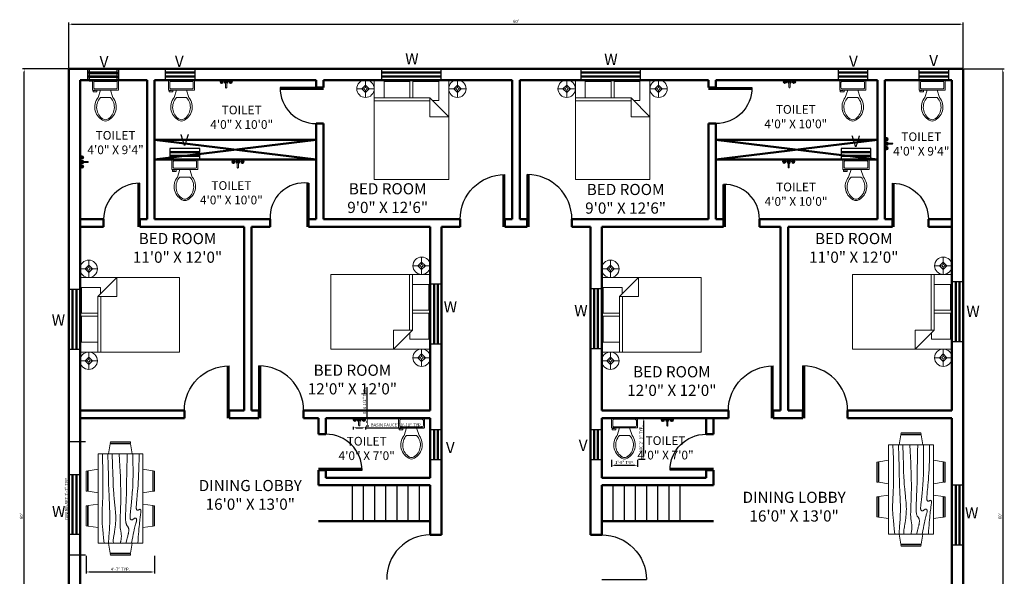
# Model space of a CAD drawing. Units: inches. Extents: x 2663 to 4539, y 2314 to 3111.
# Tile 2 of 4: x 2663 to 3456, y 2663 to 3111. Entities that reach past the tile are written whole.
import ezdxf

# ---------------------------------------------------------------- set-up
doc = ezdxf.new("R2010")
doc.units = ezdxf.units.IN
for name, color, linetype, lineweight in [('A-ANNO-DIMS', 2, 'Continuous', 18), ('A-ANNO-TEXT', 7, 'Continuous', 18), ('A-AREA-IDEN', 3, 'Continuous', 25), ('A-DOOR', 4, 'Continuous', 25), ('A-FLOR-FIXT', 8, 'Continuous', 18), ('A-FLOR-STRS', 2, 'Continuous', 25), ('A-FURN', 8, 'Continuous', 18), ('A-GLAZ', 3, 'Continuous', 25), ('A-WALL', 7, 'Continuous', 50)]:
    doc.layers.add(name, color=color, linetype=linetype, lineweight=lineweight)
doc.styles.get("Standard").update_dxf_attribs({"font": 'arial.ttf'})
doc.dimstyles.new('ISO-25', dxfattribs={"dimtxt": 2.5, "dimasz": 2.5, "dimexe": 1.25, "dimexo": 0.625, "dimtad": 1, "dimdec": 0, "dimlunit": 3, "dimtxsty": 'Standard', "dimcen": 2.5, "dimadec": 0, "dimazin": 0, "dimtfac": 1, "dimtdec": 0, "dimtmove": 0, "dimatfit": 3, "dimfxl": 1, "dimarcsym": 0})

# ---------------------------------------------------------------- blocks, each defined once
blk = doc.blocks.new('Bed - Queen')
for p, q in [((0, -80.00003), (0, 0)), ((0, 0), (59.99999, 0)), ((59.99999, 0), (59.99999, -80.00003)), ((7.99999, -1.2), (28.79998, -1.2)), ((7.99999, -14.4), (7.99999, -1.2)), ((28.79998, -1.2), (28.79998, -14.4)), ((31.19999, -1.2), (51.99999, -1.2)), ((31.19999, -14.4), (31.19999, -1.2)), ((51.99999, -1.2), (51.99999, -16.4)), ((0, -14.4), (44.8, -14.4)), ((59.99999, -29.6), (44.8, -14.4)), ((44.8, -14.4), (44.8, -29.6)), ((44.8, -16.8), (0, -16.8)), ((51.99999, -16.4), (46.79936, -16.4)), ((44.8, -29.6), (59.99999, -29.6)), ((59.99999, -80.00003), (0, -80.00003))]:
    blk.add_line(p, q)
blk = doc.blocks.new('Lamp - Table')
for p, q in [((-1, 0), (-7, 0)), ((0, 3), (-3, 0)), ((-3, 0), (0, -3)), ((0, 7), (0, 1)), ((3, 0), (0, 3)), ((0, -3), (3, 0)), ((1, 0), (7, 0)), ((0, -1), (0, -7))]:
    blk.add_line(p, q)
for radius in [7, 1]:
    blk.add_circle((0, 0), radius)
blk = doc.blocks.new('Toilet - top')
for p, q in [((9.5, -6), (9.5, -2)), ((-10, -8.5), (-8, -8.5)), ((-10, -9.5), (-10, -8.5)), ((-7, -9.5), (-10, -9.5)), ((-8, -8.5), (-8, -8)), ((-7, -8), (-7, -9.5)), ((-4, -8), (-6, -14)), ((4, -14), (-4, -14)), ((4, -8), (6, -14))]:
    blk.add_line(p, q)
blk.add_lwpolyline([(10.5, -8), (10.5, 0), (-10.5, 0), (-10.5, -8)], close=True)
for points in [[(-9.5, -2), (-9.5, -6)], [(8.5, -1), (-8.5, -1)], [(-8.5, -7), (8.5, -7)]]:
    blk.add_lwpolyline(points)
for centre, radius, start, end in [((-8.62, -1.88), 0.884, 81.8699, 188.1301), ((-8.62, -6.12), 0.884, 171.8699, 278.1301), ((8.62, -1.88), 0.884, 351.8699, 98.1301), ((8.62, -6.12), 0.884, 261.8699, 8.1301), ((3.52, -21.58), 12.17, 141.46911, 247.97143), ((4.2, -21.82), 11.33, 136.36773, 238.94682), ((-3.52, -21.58), 12.17, 292.02843, 38.53071), ((-4.2, -21.82), 11.33, 301.05301, 43.63209), ((0, -27.88), 4, 245.73182, 294.26817), ((0, -29), 4, 254.86053, 285.13947)]:
    blk.add_arc(centre, radius, start, end)
blk = doc.blocks.new('Dining Set - 36 x 72 in.')
for p, q in [((-22.2343, 26.00059), (-23.4847, 17.99762)), ((-22.2304, 26), (-5.7608, 26)), ((-22, 27.5), (-22.1562, 26.50042)), ((-5.8416, 26.5), (-22.1534, 26.5)), ((-22, 27.5), (-6, 27.5)), ((-5.8437, 26.49966), (-6, 27.5)), ((-4.5152, 17.99762), (-5.7655, 25.99926)), ((5.7657, 26.00059), (4.5153, 17.99762)), ((5.7696, 26), (22.2392, 26)), ((6, 27.5), (5.8438, 26.50042)), ((22.1584, 26.5), (5.8466, 26.5)), ((6, 27.5), (22, 27.5)), ((22.1563, 26.49966), (22, 27.5)), ((23.4848, 17.99762), (22.2345, 25.99926)), ((36, 18), (-36, 18)), ((-36, 18), (-36, -18)), ((36, -18), (36, 18)), ((-45.5, 8), (-44.5004, 8.15617)), ((-45.5, 8), (-45.5, -8)), ((-44.5, -8.15843), (-44.5, 8.15338)), ((-44.0006, 8.23428), (-35.9976, 9.48474)), ((-44, 8.23041), (-44, -8.23915)), ((44.0006, 8.23428), (35.9976, 9.48474)), ((44, 8.23041), (44, -8.23915)), ((44.5, -8.15843), (44.5, 8.15338)), ((45.5, 8), (44.5005, 8.15617)), ((45.5, 8), (45.5, -8)), ((-44.4997, -8.15631), (-45.5, -8)), ((-35.9976, -9.48476), (-43.9993, -8.2345)), ((35.9976, -9.48476), (43.9993, -8.2345)), ((44.4997, -8.15631), (45.5, -8)), ((-36, -18), (36, -18)), ((-22.2343, -26.0006), (-23.4847, -17.99762)), ((-4.5152, -17.99762), (-5.7655, -25.99928)), ((5.7657, -26.0006), (4.5153, -17.99762)), ((23.4848, -17.99762), (22.2345, -25.99928)), ((-22.2304, -26), (-5.7608, -26)), ((-22, -27.5), (-22.1562, -26.50044)), ((-5.8416, -26.5), (-22.1534, -26.5)), ((-22, -27.5), (-6, -27.5)), ((-5.8437, -26.49967), (-6, -27.5)), ((5.7696, -26), (22.2392, -26)), ((6, -27.5), (5.8438, -26.50044)), ((22.1584, -26.5), (5.8466, -26.5)), ((6, -27.5), (22, -27.5)), ((22.1563, -26.49967), (22, -27.5))]:
    blk.add_line(p, q)
for points in [[(-36, 15), (-31.1772, 14.97754), (-26.8079, 14.91406), (-22.8538, 14.81543), (-19.276, 14.6875), (-16.0362, 14.53613), (-13.0957, 14.36718), (-10.4159, 14.18652), (-7.9583, 14), (-5.6904, 13.81315), (-3.6035, 13.63021), (-1.6954, 13.45508), (0.0365, 13.29166), (1.5945, 13.14388), (2.9811, 13.01562), (4.1988, 12.9108), (5.25, 12.83333), (6.1393, 12.78613), (6.8802, 12.76823), (7.4883, 12.77767), (7.9792, 12.8125), (8.3685, 12.87077), (8.6719, 12.95052), (8.9049, 13.0498), (9.0833, 13.16666), (9.2205, 13.29899), (9.3216, 13.44401), (9.3895, 13.59879), (9.4271, 13.76041), (9.4373, 13.92594), (9.4232, 14.09245), (9.3875, 14.257), (9.3333, 14.41666), (9.2638, 14.56917), (9.1836, 14.71484), (9.0975, 14.85465), (9.0104, 14.98958), (8.9272, 15.1206), (8.8529, 15.2487), (8.7922, 15.37483), (8.75, 15.5), (8.7305, 15.62467), (8.7344, 15.74739), (8.7617, 15.86621), (8.8125, 15.97916), (8.8867, 16.08431), (8.9844, 16.17968), (9.1055, 16.26334), (9.25, 16.33333), (9.4189, 16.38802), (9.6172, 16.42708), (9.8506, 16.45052), (10.125, 16.45833), (10.4463, 16.45052), (10.8203, 16.42708), (11.2529, 16.38802), (11.75, 16.33333), (12.3184, 16.26318), (12.9694, 16.17838), (13.7151, 16.07991), (14.5677, 15.96875), (15.5395, 15.84586), (16.6426, 15.71224), (17.8893, 15.56884), (19.2917, 15.41666), (20.859, 15.25667), (22.5879, 15.08984), (24.4721, 14.91715), (26.5052, 14.73958), (28.6809, 14.5581), (30.9929, 14.3737), (33.4347, 14.18733), (36, 14)], [(-36, 10), (-28.9766, 10.14274), (-23.1725, 10.20442), (-18.4241, 10.19775), (-14.5677, 10.13541), (-11.4399, 10.03011), (-8.877, 9.89453), (-6.7154, 9.74137), (-4.7917, 9.58333), (-2.9698, 9.43082), (-1.2246, 9.28515), (0.4415, 9.14534), (2.026, 9.01041), (3.5266, 8.87939), (4.9408, 8.7513), (6.266, 8.62516), (7.5, 8.5), (8.6411, 8.37549), (9.6914, 8.2539), (10.6538, 8.13818), (11.5312, 8.03125), (12.3267, 7.93603), (13.043, 7.85547), (13.6831, 7.79248), (14.25, 7.75), (14.7471, 7.7303), (15.1797, 7.73307), (15.5537, 7.75732), (15.875, 7.80208), (16.1494, 7.86637), (16.3828, 7.94922), (16.5811, 8.04964), (16.75, 8.16666), (16.8944, 8.29915), (17.0143, 8.44531), (17.1089, 8.60319), (17.1771, 8.77083), (17.218, 8.94629), (17.2305, 9.1276), (17.2137, 9.31282), (17.1667, 9.5), (17.0895, 9.6875), (16.987, 9.875), (16.8649, 10.0625), (16.7292, 10.25), (16.5856, 10.4375), (16.4401, 10.625), (16.2985, 10.8125), (16.1667, 11), (16.05, 11.18733), (15.9518, 11.3737), (15.8752, 11.5581), (15.8229, 11.73958), (15.798, 11.91715), (15.8034, 12.08984), (15.842, 12.25667), (15.9167, 12.41666), (16.0295, 12.56836), (16.1784, 12.70833), (16.3605, 12.83268), (16.5729, 12.9375), (16.8127, 13.01888), (17.0768, 13.07291), (17.3625, 13.0957), (17.6667, 13.08333), (17.9894, 13.03312), (18.3418, 12.94726), (18.7382, 12.82918), (19.1927, 12.68229), (19.7195, 12.51001), (20.3327, 12.31575), (21.0465, 12.10294), (21.875, 11.875), (22.8357, 11.63354), (23.959, 11.37304), (25.2786, 11.08618), (26.8282, 10.76562), (28.6414, 10.40405), (30.752, 9.99414), (33.1936, 9.52856), (36, 9)], [(-36, 5.5), (-30.7157, 5.3348), (-26.069, 5.20963), (-21.9946, 5.11767), (-18.4271, 5.05208), (-15.3009, 5.00602), (-12.5508, 4.97265), (-10.1112, 4.94515), (-7.9167, 4.91666), (-5.909, 4.88167), (-4.0586, 4.83984), (-2.3429, 4.79215), (-0.7396, 4.73958), (0.7739, 4.6831), (2.22, 4.6237), (3.6213, 4.56233), (5, 4.5), (6.373, 4.43782), (7.7344, 4.3776), (9.0723, 4.32129), (10.375, 4.27083), (11.6309, 4.22819), (12.8281, 4.19531), (13.9551, 4.17415), (15, 4.16666), (15.954, 4.17448), (16.819, 4.19791), (17.6001, 4.23698), (18.3021, 4.29166), (18.9299, 4.36198), (19.4883, 4.44791), (19.9823, 4.54948), (20.4167, 4.66666), (20.7969, 4.79899), (21.1302, 4.94401), (21.4245, 5.09879), (21.6875, 5.26041), (21.9271, 5.42594), (22.1511, 5.59245), (22.3672, 5.757), (22.5834, 5.91666), (22.8065, 6.06868), (23.0404, 6.21093), (23.2879, 6.34147), (23.5521, 6.45833), (23.8358, 6.55957), (24.142, 6.64323), (24.4735, 6.70735), (24.8334, 6.75), (25.2235, 6.76969), (25.642, 6.76692), (26.0858, 6.74267), (26.5521, 6.69791), (27.0379, 6.63362), (27.5404, 6.55078), (28.0565, 6.45036), (28.5834, 6.33333), (29.1242, 6.19987), (29.7071, 6.04687), (30.3661, 5.87044), (31.1354, 5.66666), (32.0493, 5.43164), (33.142, 5.16146), (34.4475, 4.85221), (36, 4.5)], [(-36, -1), (-30.7915, -0.6591), (-26.0195, -0.38216), (-21.6519, -0.16284), (-17.6563, 0.00521), (-14.0005, 0.12833), (-10.6523, 0.21289), (-7.5796, 0.26522), (-4.75, 0.29166), (-2.134, 0.29793), (0.2878, 0.28711), (2.5317, 0.26163), (4.6146, 0.22396), (6.5529, 0.17651), (8.3633, 0.12174), (10.0623, 0.06209), (11.6667, 0), (13.1899, -0.06201), (14.6341, -0.1211), (15.9982, -0.17432), (17.2813, -0.21875), (18.4823, -0.25147), (19.6003, -0.26953), (20.6343, -0.27002), (21.5834, -0.25), (22.4481, -0.20768), (23.2357, -0.14584), (23.9549, -0.06836), (24.6146, 0.02083), (25.2235, 0.11784), (25.7904, 0.21875), (26.3241, 0.31966), (26.8334, 0.41666), (27.3265, 0.50618), (27.8099, 0.58593), (28.2894, 0.65397), (28.7709, 0.70833), (29.2601, 0.74707), (29.763, 0.76823), (30.2855, 0.76985), (30.8334, 0.75), (31.4088, 0.70784), (31.9994, 0.64713), (32.589, 0.57275), (33.1615, 0.48958), (33.7008, 0.4025), (34.1908, 0.3164), (34.6153, 0.23616), (34.9584, 0.16666), (35.2099, 0.11165), (35.3848, 0.07031), (35.504, 0.04069), (35.5886, 0.02083), (35.6594, 0.00879), (35.7377, 0.0026), (35.8442, 0.00032), (36, 0)], [(-36, -6.5), (-27.1843, -6.31267), (-20.084, -6.1263), (-14.469, -5.9419), (-10.1094, -5.76042), (-6.7752, -5.58285), (-4.2363, -5.41016), (-2.2629, -5.24333), (-0.625, -5.08334), (0.8708, -4.93099), (2.2715, -4.78646), (3.5872, -4.64974), (4.8281, -4.52084), (6.0046, -4.39974), (7.127, -4.28646), (8.2053, -4.18099), (9.25, -4.08334), (10.2705, -3.99382), (11.2734, -3.91407), (12.2647, -3.84603), (13.25, -3.79167), (14.2354, -3.75293), (15.2266, -3.73177), (16.2295, -3.73015), (17.25, -3.75), (18.2912, -3.79248), (19.3451, -3.85547), (20.4009, -3.93604), (21.4479, -4.03125), (22.4754, -4.13819), (23.4727, -4.25391), (24.4289, -4.37549), (25.3334, -4.5), (26.1785, -4.62492), (26.9694, -4.74935), (27.7145, -4.87281), (28.4219, -4.99479), (29.1, -5.11483), (29.7572, -5.23242), (30.4016, -5.34709), (31.0417, -5.45834), (31.6837, -5.56437), (32.3262, -5.65821), (32.9658, -5.73153), (33.599, -5.77604), (34.2224, -5.78345), (34.8327, -5.74545), (35.4264, -5.65373), (36, -5.5)], [(-36, -10), (-26.4022, -9.81299), (-18.4675, -9.62891), (-11.9839, -9.45069), (-6.7396, -9.28125), (-2.5226, -9.12354), (0.8789, -8.98047), (3.6769, -8.85498), (6.0833, -8.75), (8.2767, -8.66765), (10.3021, -8.60677), (12.1712, -8.56543), (13.8958, -8.54167), (15.4876, -8.53353), (16.9583, -8.53907), (18.3197, -8.55632), (19.5834, -8.58334), (20.7616, -8.61841), (21.8685, -8.66081), (22.9188, -8.71004), (23.9271, -8.76563), (24.9081, -8.82707), (25.8763, -8.89388), (26.8465, -8.96558), (27.8334, -9.04167), (28.8474, -9.12118), (29.8828, -9.20117), (30.93, -9.27824), (31.9792, -9.34896), (33.0205, -9.40991), (34.0443, -9.45768), (35.0407, -9.48885), (36, -9.5)], [(-36, -14.5), (-30.0881, -14.33513), (-25.0332, -14.21224), (-20.7312, -14.12647), (-17.0781, -14.07292), (-13.97, -14.04671), (-11.3027, -14.04297), (-8.9724, -14.05681), (-6.875, -14.08334), (-4.9224, -14.11833), (-3.0905, -14.16016), (-1.3709, -14.20785), (0.2448, -14.26042), (1.7647, -14.3169), (3.1973, -14.3763), (4.5507, -14.43767), (5.8333, -14.5), (7.0554, -14.5621), (8.235, -14.62175), (9.3922, -14.67652), (10.5469, -14.72396), (11.7192, -14.76164), (12.929, -14.78711), (14.1965, -14.79794), (15.5417, -14.79167), (16.9933, -14.76424), (18.6152, -14.70508), (20.4804, -14.60197), (22.6615, -14.44271), (25.2312, -14.21509), (28.2624, -13.9069), (31.8277, -13.50594), (36, -13)]]:
    blk.add_lwpolyline(points)
blk = doc.blocks.new('Faucet - Bathroom top')
for p, q in [((-4.107, 0.125), (-4.375, 0.125)), ((-3.75, 0.4788), (-3.75, 0.75)), ((-3.5, 0.482), (-3.5, 0.75)), ((-3.1461, 0.125), (-2.875, 0.125)), ((3.143, 0.125), (2.875, 0.125)), ((3.5, 0.4788), (3.5, 0.75)), ((3.75, 0.482), (3.75, 0.75)), ((4.1039, 0.125), (4.375, 0.125)), ((-4.1039, -0.125), (-4.375, -0.125)), ((-3.75, -0.4821), (-3.75, -0.75)), ((-3.5, -0.4789), (-3.5, -0.75)), ((-3.143, -0.125), (-2.875, -0.125)), ((-0.5, -0.8639), (-0.5, -4.5)), ((0.5, -4.5), (0.5, -0.8631)), ((3.1461, -0.125), (2.875, -0.125)), ((3.5, -0.4821), (3.5, -0.75)), ((3.75, -0.4789), (3.75, -0.75)), ((4.107, -0.125), (4.375, -0.125))]:
    blk.add_line(p, q)
for centre, radius in [((-3.625, 0), 1.375), ((-4.625, 0), 0.2795), ((-3.625, 0), 0.5), ((-3.625, 1), 0.2795), ((-2.625, 0), 0.2795), ((0, 0), 0.5), ((3.625, 0), 1.375), ((2.625, 0), 0.2795), ((3.625, 0), 0.5), ((3.625, 1), 0.2795), ((4.625, 0), 0.2795), ((-3.625, -1), 0.2795), ((3.625, -1), 0.2795)]:
    blk.add_circle(centre, radius)
for centre, radius, start, end in [((-3.625, 0), 1, 105.2407, 164.2093), ((-3.625, 0), 1, 16.44125, 74.07887), ((0, 0), 1.5, 289.6514, 250.3603), ((0, 0), 1, 300.3431, 239.7554), ((3.625, 0), 1, 106.12, 164.0884), ((3.625, 0), 1, 16.23422, 73.90469), ((-3.625, 0), 1, 196.2342, 253.9047), ((-3.625, 0), 1, 286.12, 344.0884), ((0, -4.5), 0.5, 180, 0), ((3.625, 0), 1, 196.4413, 254.0789), ((3.625, 0), 1, 285.2407, 344.2093)]:
    blk.add_arc(centre, radius, start, end)
blk = doc.blocks.new('*D10')
at = {"layer": 'A-ANNO-DIMS', "color": 0, "lineweight": -2, "transparency": 16777216}
for p, q in [((2702.63, 3071.54), (2702.63, 3108.16)), ((3422.63, 3071.54), (3422.63, 3108.16)), ((2705.13, 3106.91), (3420.13, 3106.91))]:
    blk.add_line(p, q, dxfattribs=at)
at = {"layer": 'A-ANNO-DIMS', "color": 0, "transparency": 16777216}
for points in [[(2705.13, 3107.33), (2705.13, 3106.5), (2702.63, 3106.91)], [(3420.13, 3107.33), (3420.13, 3106.5), (3422.63, 3106.91)]]:
    blk.add_solid(points, dxfattribs=at)
at = {"layer": 'Defpoints', "color": 0, "transparency": 16777216}
for p in [(3422.63, 3106.91), (2702.63, 3070.91), (3422.63, 3070.91)]:
    blk.add_point(p, dxfattribs=at)
at = {"layer": 'A-ANNO-DIMS', "color": 0, "transparency": 16777216, "insert": (3062.63, 3108.82), "char_height": 2.5, "attachment_point": 5}
blk.add_mtext("60'", dxfattribs=at)
blk = doc.blocks.new('*D11')
at = {"layer": 'A-ANNO-DIMS', "color": 0, "lineweight": -2, "transparency": 16777216}
for p, q in [((3423.26, 3070.91), (3455.77, 3070.91)), ((3454.52, 3068.41), (3454.52, 2353.41)), ((3423.26, 2350.91), (3455.77, 2350.91))]:
    blk.add_line(p, q, dxfattribs=at)
at = {"layer": 'A-ANNO-DIMS', "color": 0, "transparency": 16777216}
for points in [[(3454.11, 3068.41), (3454.94, 3068.41), (3454.52, 3070.91)], [(3454.11, 2353.41), (3454.94, 2353.41), (3454.52, 2350.91)]]:
    blk.add_solid(points, dxfattribs=at)
at = {"layer": 'Defpoints', "color": 0, "transparency": 16777216}
for p in [(3422.63, 3070.91), (3422.63, 2350.91), (3454.52, 2350.91)]:
    blk.add_point(p, dxfattribs=at)
at = {"layer": 'A-ANNO-DIMS', "color": 0, "transparency": 16777216, "insert": (3452.62, 2710.91), "char_height": 2.5, "attachment_point": 5, "rotation": 90}
blk.add_mtext("60'", dxfattribs=at)
blk = doc.blocks.new('*D19')
at = {"layer": 'A-ANNO-DIMS', "color": 0, "lineweight": -2, "transparency": 16777216}
for p, q in [((2702.01, 3070.91), (2665.38, 3070.91)), ((2666.63, 2353.41), (2666.63, 3068.41)), ((2702.01, 2350.91), (2665.38, 2350.91))]:
    blk.add_line(p, q, dxfattribs=at)
at = {"layer": 'A-ANNO-DIMS', "color": 0, "transparency": 16777216}
for points in [[(2666.21, 3068.41), (2667.05, 3068.41), (2666.63, 3070.91)], [(2666.21, 2353.41), (2667.05, 2353.41), (2666.63, 2350.91)]]:
    blk.add_solid(points, dxfattribs=at)
at = {"layer": 'Defpoints', "color": 0, "transparency": 16777216}
for p in [(2666.63, 3070.91), (2702.63, 3070.91), (2702.63, 2350.91)]:
    blk.add_point(p, dxfattribs=at)
at = {"layer": 'A-ANNO-DIMS', "color": 0, "transparency": 16777216, "insert": (2664.73, 2710.91), "char_height": 2.5, "attachment_point": 5, "rotation": 90}
blk.add_mtext("60'", dxfattribs=at)
blk = doc.blocks.new('WIN-1200')
for p, q in [((0, 48), (0, 0)), ((9, 48), (0, 48)), ((0, 48), (0, 48)), ((9, 0), (9, 48)), ((0, 0), (9, 0))]:
    blk.add_line(p, q)
blk = doc.blocks.new('VENT-600')
for p, q in [((24, 9), (0, 9)), ((0, 9), (0, 0)), ((24, 0), (24, 9)), ((0, 0), (24, 0))]:
    blk.add_line(p, q)
blk = doc.blocks.new('DOOR-750')
blk.add_line((2901.63, 3055.91), (2872.63, 3055.91))
blk.add_arc((2901.63, 3055.91), 29, 180, 270)
blk = doc.blocks.new('DOOR-900')
blk.add_line((3071.63, 2949.91), (3071.63, 2985.91))
blk.add_arc((3071.63, 2949.91), 36, 0, 90)
blk = doc.blocks.new('*D32')
at = {"layer": 'A-ANNO-DIMS', "color": 0, "lineweight": -2, "transparency": 16777216}
for p, q in [((3161.16, 2789.91), (3166.74, 2789.91)), ((3165.49, 2759.37), (3165.49, 2787.41)), ((3161.16, 2756.87), (3166.74, 2756.87))]:
    blk.add_line(p, q, dxfattribs=at)
at = {"layer": 'A-ANNO-DIMS', "color": 0, "transparency": 16777216}
for points in [[(3165.07, 2787.41), (3165.91, 2787.41), (3165.49, 2789.91)], [(3165.07, 2759.37), (3165.91, 2759.37), (3165.49, 2756.87)]]:
    blk.add_solid(points, dxfattribs=at)
at = {"layer": 'Defpoints', "color": 0, "transparency": 16777216}
for p in [(3160.53, 2789.91), (3165.49, 2789.91), (3160.53, 2756.87)]:
    blk.add_point(p, dxfattribs=at)
at = {"layer": 'A-ANNO-DIMS', "color": 0, "transparency": 16777216, "insert": (3163.57, 2773.39), "char_height": 2.5, "attachment_point": 5, "rotation": 90}
blk.add_mtext('WC 2\'-9" TYP.', dxfattribs=at)
blk = doc.blocks.new('*D33')
at = {"layer": 'A-ANNO-DIMS', "color": 0, "lineweight": -2, "transparency": 16777216}
for p, q in [((3139.53, 2756.24), (3139.53, 2750.66)), ((3142.03, 2751.91), (3158.03, 2751.91)), ((3160.53, 2756.24), (3160.53, 2750.66))]:
    blk.add_line(p, q, dxfattribs=at)
at = {"layer": 'A-ANNO-DIMS', "color": 0, "transparency": 16777216}
for points in [[(3142.03, 2752.33), (3142.03, 2751.5), (3139.53, 2751.91)], [(3158.03, 2752.33), (3158.03, 2751.5), (3160.53, 2751.91)]]:
    blk.add_solid(points, dxfattribs=at)
at = {"layer": 'Defpoints', "color": 0, "transparency": 16777216}
for p in [(3139.53, 2756.87), (3160.53, 2756.87), (3160.53, 2751.91)]:
    blk.add_point(p, dxfattribs=at)
at = {"layer": 'A-ANNO-DIMS', "color": 0, "transparency": 16777216, "insert": (3150.03, 2753.81), "char_height": 2.5, "attachment_point": 5}
blk.add_mtext('1\'-9" TYP.', dxfattribs=at)
blk = doc.blocks.new('*D34')
at = {"layer": 'A-ANNO-DIMS', "color": 0, "lineweight": -2, "transparency": 16777216}
for p, q in [((2931.42, 2782.93), (2931.42, 2780.81)), ((2941.42, 2782.93), (2941.42, 2780.81)), ((2933.92, 2782.06), (2938.92, 2782.06)), ((2941.42, 2782.06), (2988.63, 2782.06))]:
    blk.add_line(p, q, dxfattribs=at)
at = {"layer": 'A-ANNO-DIMS', "color": 0, "transparency": 16777216}
for points in [[(2933.92, 2782.48), (2933.92, 2781.64), (2931.42, 2782.06)], [(2938.92, 2782.48), (2938.92, 2781.64), (2941.42, 2782.06)]]:
    blk.add_solid(points, dxfattribs=at)
at = {"layer": 'Defpoints', "color": 0, "transparency": 16777216}
for p in [(2931.42, 2783.56), (2941.42, 2783.56), (2941.42, 2782.06)]:
    blk.add_point(p, dxfattribs=at)
at = {"layer": 'A-ANNO-DIMS', "color": 0, "transparency": 16777216, "insert": (2966.28, 2783.98), "char_height": 2.5, "attachment_point": 5}
blk.add_mtext('BASIN FAUCET 0\'-10" TYP.', dxfattribs=at)
blk = doc.blocks.new('*D35')
at = {"layer": 'A-ANNO-DIMS', "color": 0, "lineweight": -2, "transparency": 16777216}
for p, q in [((2942.92, 2790.06), (2942.92, 2814.87)), ((2942.05, 2790.06), (2944.17, 2790.06)), ((2942.05, 2783.56), (2944.17, 2783.56)), ((2942.92, 2786.06), (2942.92, 2787.56))]:
    blk.add_line(p, q, dxfattribs=at)
at = {"layer": 'A-ANNO-DIMS', "color": 0, "transparency": 16777216}
for points in [[(2942.5, 2787.56), (2943.34, 2787.56), (2942.92, 2790.06)], [(2942.5, 2786.06), (2943.34, 2786.06), (2942.92, 2783.56)]]:
    blk.add_solid(points, dxfattribs=at)
at = {"layer": 'Defpoints', "color": 0, "transparency": 16777216}
for p in [(2941.42, 2790.06), (2941.42, 2783.56), (2942.92, 2790.06)]:
    blk.add_point(p, dxfattribs=at)
at = {"layer": 'A-ANNO-DIMS', "color": 0, "transparency": 16777216, "insert": (2941, 2803.72), "char_height": 2.5, "attachment_point": 5, "rotation": 90}
blk.add_mtext('0\'-6 1/2" TYP.', dxfattribs=at)
blk = doc.blocks.new('*D44')
at = {"layer": 'A-ANNO-DIMS', "color": 0, "lineweight": -2, "transparency": 16777216}
for p, q in [((2715.98, 2770.68), (2701.71, 2770.68)), ((2702.96, 2768.18), (2702.96, 2682.18)), ((2715.98, 2679.68), (2701.71, 2679.68))]:
    blk.add_line(p, q, dxfattribs=at)
at = {"layer": 'A-ANNO-DIMS', "color": 0, "transparency": 16777216}
for points in [[(2702.54, 2768.18), (2703.38, 2768.18), (2702.96, 2770.68)], [(2702.54, 2682.18), (2703.38, 2682.18), (2702.96, 2679.68)]]:
    blk.add_solid(points, dxfattribs=at)
at = {"layer": 'Defpoints', "color": 0, "transparency": 16777216}
for p in [(2716.61, 2770.68), (2702.96, 2679.68), (2716.61, 2679.68)]:
    blk.add_point(p, dxfattribs=at)
at = {"layer": 'A-ANNO-DIMS', "color": 0, "transparency": 16777216, "insert": (2701.04, 2725.18), "char_height": 2.5, "attachment_point": 5, "rotation": 90}
blk.add_mtext('DINING SET 7\'-7" TYP.', dxfattribs=at)
blk = doc.blocks.new('*D45')
at = {"layer": 'A-ANNO-DIMS', "color": 0, "lineweight": -2, "transparency": 16777216}
for p, q in [((2716.61, 2679.05), (2716.61, 2664.78)), ((2771.61, 2679.05), (2771.61, 2664.78)), ((2719.11, 2666.03), (2769.11, 2666.03))]:
    blk.add_line(p, q, dxfattribs=at)
at = {"layer": 'A-ANNO-DIMS', "color": 0, "transparency": 16777216}
for points in [[(2719.11, 2666.45), (2719.11, 2665.61), (2716.61, 2666.03)], [(2769.11, 2666.45), (2769.11, 2665.61), (2771.61, 2666.03)]]:
    blk.add_solid(points, dxfattribs=at)
at = {"layer": 'Defpoints', "color": 0, "transparency": 16777216}
for p in [(2716.61, 2679.68), (2771.61, 2679.68), (2771.61, 2666.03)]:
    blk.add_point(p, dxfattribs=at)
at = {"layer": 'A-ANNO-DIMS', "color": 0, "transparency": 16777216, "insert": (2744.11, 2667.91), "char_height": 2.5, "attachment_point": 5}
blk.add_mtext('4\'-7" TYP.', dxfattribs=at)

msp = doc.modelspace()

# ---------------------------------------------------------------- linework, layer by layer
at = {"layer": 'A-DOOR'}
for centre, radius, start, end in [((2892.16, 2951.55), 27.58, 82.77506, 183.40664), ((3230.63, 2949.91), 28, 360, 92.04671), ((2993.63, 2660.91), 35, 90, 181.63725)]:
    msp.add_arc(centre, radius, start, end, dxfattribs=at)
at = {"layer": 'A-FLOR-STRS'}
for p, q in [((2930.63, 2735.91), (2930.63, 2706.91)), ((2939.63, 2735.91), (2939.63, 2706.91)), ((2948.63, 2735.91), (2948.63, 2706.91)), ((2957.63, 2735.91), (2957.63, 2706.91)), ((2966.63, 2735.91), (2966.63, 2706.91)), ((2975.63, 2735.91), (2975.63, 2706.91)), ((2984.63, 2735.91), (2984.63, 2706.91)), ((3140.63, 2735.91), (3140.63, 2706.91)), ((3149.63, 2735.91), (3149.63, 2706.91)), ((3158.63, 2735.91), (3158.63, 2706.91)), ((3167.63, 2735.91), (3167.63, 2706.91)), ((3176.63, 2735.91), (3176.63, 2706.91)), ((3185.63, 2735.91), (3185.63, 2706.91)), ((3194.63, 2735.91), (3194.63, 2706.91))]:
    msp.add_line(p, q, dxfattribs=at)
at = {"layer": 'A-WALL'}
for p, q in [((2702.63, 3070.91), (3422.63, 3070.91)), ((2702.63, 2350.91), (2702.63, 3070.91)), ((3422.63, 3070.91), (3422.63, 2350.91)), ((2711.63, 3061.91), (2765.63, 3061.91)), ((2711.63, 2624.91), (2711.63, 3061.91)), ((2741.59, 3067.91), (2717.59, 3067.91)), ((2717.59, 3064.91), (2741.59, 3064.91)), ((2742.88, 3067.41), (2718.88, 3067.41)), ((2718.88, 3064.41), (2742.88, 3064.41)), ((2765.63, 2949.91), (2765.63, 3061.91)), ((2771.63, 2949.91), (2771.63, 3061.91)), ((2771.63, 3061.91), (2901.63, 3061.91)), ((2804.19, 3067.91), (2780.19, 3067.91)), ((2780.19, 3064.91), (2804.19, 3064.91)), ((2901.63, 3061.91), (2901.63, 3055.91)), ((2901.63, 3055.91), (2901.63, 3061.91)), ((2907.63, 3061.91), (3059.63, 3061.91)), ((2907.63, 3055.91), (2907.63, 3061.91)), ((3002.32, 3067.91), (2954.32, 3067.91)), ((2954.32, 3064.91), (3002.32, 3064.91)), ((3059.63, 2949.91), (3059.63, 3061.91)), ((3065.63, 3061.91), (3065.63, 2949.91)), ((3065.63, 3061.91), (3217.63, 3061.91)), ((3162.93, 3067.91), (3114.93, 3067.91)), ((3114.93, 3064.91), (3162.93, 3064.91)), ((3217.63, 3061.91), (3217.63, 3055.91)), ((3223.63, 3061.91), (3223.63, 3055.91)), ((3223.63, 3061.91), (3353.63, 3061.91)), ((3223.63, 3061.91), (3223.63, 3055.91)), ((3345.92, 3067.91), (3321.92, 3067.91)), ((3321.92, 3064.91), (3345.92, 3064.91)), ((3353.63, 3061.91), (3353.63, 2949.91)), ((3359.63, 3061.91), (3359.63, 2949.91)), ((3359.63, 3061.91), (3413.63, 3061.91)), ((3411.01, 3067.91), (3387.01, 3067.91)), ((3387.01, 3064.91), (3411.01, 3064.91)), ((3413.63, 3061.91), (3413.63, 2795.91)), ((2901.63, 3054.91), (2872.63, 3054.91)), ((2901.63, 3055.91), (2907.63, 3055.91)), ((2901.63, 3054.91), (2907.63, 3054.91)), ((3223.63, 3055.91), (3217.63, 3055.91)), ((3223.63, 3054.91), (3217.63, 3054.91)), ((3223.63, 3054.91), (3252.63, 3054.91)), ((2901.63, 2949.91), (2901.63, 3026.91)), ((2907.63, 3026.91), (2901.63, 3026.91)), ((2907.63, 2949.91), (2907.63, 3026.91)), ((3217.63, 3026.91), (3223.63, 3026.91)), ((3217.63, 3026.91), (3217.63, 2949.91)), ((3223.63, 3026.91), (3223.63, 2949.91)), ((2771.63, 3013.91), (2901.63, 3013.91)), ((2771.63, 3013.91), (2901.63, 2997.91)), ((2901.63, 3013.91), (2771.63, 2997.91)), ((2901.63, 2997.91), (2901.63, 3013.91)), ((3223.63, 3013.91), (3353.63, 3013.91)), ((3353.63, 3013.91), (3223.63, 2997.91)), ((3223.63, 2997.91), (3223.63, 3013.91)), ((3223.63, 3013.91), (3353.63, 2997.91)), ((2771.63, 2997.91), (2901.63, 2997.91)), ((2808.04, 3003.94), (2784.04, 3003.94)), ((2784.04, 3000.94), (2808.04, 3000.94)), ((3223.63, 2997.91), (3353.63, 2997.91)), ((3348.36, 3003.88), (3324.36, 3003.88)), ((3324.36, 3000.88), (3348.36, 3000.88)), ((3052.63, 2949.91), (3052.63, 2985.91)), ((3072.63, 2949.91), (3072.63, 2985.91)), ((2758.63, 2949.91), (2758.63, 2978.91)), ((2894.63, 2949.91), (2894.63, 2978.91)), ((2895.63, 2949.91), (2895.63, 2978.91)), ((3229.63, 2949.91), (3229.63, 2977.9)), ((3230.63, 2949.91), (3230.63, 2977.91)), ((3366.63, 2949.91), (3366.63, 2978.91)), ((2711.63, 2949.91), (2730.63, 2949.91)), ((2730.63, 2943.91), (2730.63, 2949.91)), ((2758.63, 2949.91), (2758.63, 2943.91)), ((2765.63, 2949.91), (2759.63, 2949.91)), ((2759.63, 2949.91), (2759.63, 2943.91)), ((2759.63, 2949.91), (2765.63, 2949.91)), ((2771.63, 2949.91), (2864.63, 2949.91)), ((2864.63, 2943.91), (2864.63, 2949.91)), ((2894.63, 2949.91), (2894.63, 2943.91)), ((2901.63, 2949.91), (2895.63, 2949.91)), ((2895.63, 2949.91), (2895.63, 2943.91)), ((2895.63, 2949.91), (2901.63, 2949.91)), ((2907.63, 2949.91), (3017.63, 2949.91)), ((3017.63, 2943.91), (3017.63, 2949.91)), ((3052.63, 2949.91), (3052.63, 2943.91)), ((3059.63, 2949.91), (3053.63, 2949.91)), ((3053.63, 2949.91), (3053.63, 2943.91)), ((3053.63, 2949.91), (3059.63, 2949.91)), ((3065.63, 2949.91), (3071.63, 2949.91)), ((3065.63, 2949.91), (3071.63, 2949.91)), ((3071.63, 2949.91), (3071.63, 2943.91)), ((3072.63, 2949.91), (3072.63, 2943.91)), ((3107.63, 2943.91), (3107.63, 2949.91)), ((3107.63, 2949.91), (3217.63, 2949.91)), ((3223.63, 2949.91), (3229.63, 2949.91)), ((3223.63, 2949.91), (3229.63, 2949.91)), ((3229.63, 2949.91), (3229.63, 2943.91)), ((3230.63, 2949.91), (3230.63, 2943.91)), ((3258.63, 2943.91), (3258.63, 2949.91)), ((3258.63, 2949.91), (3353.63, 2949.91)), ((3359.63, 2949.91), (3365.63, 2949.91)), ((3359.63, 2949.91), (3365.63, 2949.91)), ((3365.63, 2949.91), (3365.63, 2943.91)), ((3366.63, 2949.91), (3366.63, 2943.91)), ((3394.63, 2943.91), (3394.63, 2949.91)), ((3394.63, 2949.91), (3413.63, 2949.91)), ((2711.63, 2943.91), (2730.63, 2943.91)), ((2759.63, 2943.91), (2843.63, 2943.91)), ((2843.63, 2795.91), (2843.63, 2943.91)), ((2849.63, 2795.91), (2849.63, 2943.91)), ((2849.63, 2943.91), (2864.63, 2943.91)), ((2895.63, 2943.91), (2993.63, 2943.91)), ((2993.63, 2795.91), (2993.63, 2943.91)), ((3002.63, 2943.91), (3017.63, 2943.91)), ((3002.63, 2795.91), (3002.63, 2943.91)), ((3053.63, 2943.91), (3071.63, 2943.91)), ((3107.63, 2943.91), (3122.63, 2943.91)), ((3122.63, 2943.91), (3122.63, 2795.91)), ((3131.63, 2943.91), (3131.63, 2795.91)), ((3131.63, 2943.91), (3229.63, 2943.91)), ((3258.63, 2943.91), (3275.63, 2943.91)), ((3275.63, 2943.91), (3275.63, 2795.91)), ((3281.63, 2943.91), (3281.63, 2795.91)), ((3281.63, 2943.91), (3365.63, 2943.91)), ((3394.63, 2943.91), (3413.63, 2943.91)), ((2996.63, 2897.72), (2996.63, 2849.72)), ((2999.63, 2849.72), (2999.63, 2897.72)), ((3125.63, 2893.91), (3125.63, 2845.91)), ((3128.63, 2845.91), (3128.63, 2893.91)), ((3416.63, 2899.47), (3416.63, 2851.47)), ((3419.63, 2851.47), (3419.63, 2899.47)), ((2705.63, 2893.48), (2705.63, 2845.48)), ((2708.63, 2845.48), (2708.63, 2893.48)), ((2830.63, 2795.91), (2830.63, 2831.91)), ((2856.63, 2795.91), (2856.63, 2831.91)), ((3268.63, 2795.91), (3268.63, 2831.91)), ((3294.63, 2795.91), (3294.63, 2831.91)), ((2711.63, 2795.91), (2795.63, 2795.91)), ((2795.63, 2789.91), (2795.63, 2795.91)), ((2830.63, 2795.91), (2830.63, 2789.91)), ((2837.63, 2795.91), (2831.63, 2795.91)), ((2843.63, 2795.91), (2831.63, 2795.91)), ((2831.63, 2795.91), (2831.63, 2789.91)), ((2843.63, 2795.91), (2837.63, 2795.91)), ((2837.63, 2795.91), (2843.63, 2795.91)), ((2849.63, 2795.91), (2855.63, 2795.91)), ((2849.63, 2795.91), (2855.63, 2795.91)), ((2855.63, 2795.91), (2855.63, 2789.91)), ((2856.63, 2795.91), (2856.63, 2789.91)), ((2891.63, 2789.91), (2891.63, 2795.91)), ((2891.63, 2795.91), (2993.63, 2795.91)), ((3002.63, 2795.91), (3002.63, 2695.91)), ((3122.63, 2795.91), (3122.63, 2695.91)), ((3131.63, 2795.91), (3233.63, 2795.91)), ((3233.63, 2789.91), (3233.63, 2795.91)), ((3268.63, 2795.91), (3268.63, 2789.91)), ((3275.63, 2795.91), (3269.63, 2795.91)), ((3269.63, 2795.91), (3269.63, 2789.91)), ((3269.63, 2795.91), (3275.63, 2795.91)), ((3281.63, 2795.91), (3293.63, 2795.91)), ((3281.63, 2795.91), (3293.63, 2795.91)), ((3293.63, 2795.91), (3293.63, 2789.91)), ((3294.63, 2795.91), (3294.63, 2789.91)), ((3329.63, 2789.91), (3329.63, 2795.91)), ((3329.63, 2795.91), (3413.63, 2795.91)), ((2711.63, 2789.91), (2795.63, 2789.91)), ((2837.63, 2789.91), (2831.63, 2789.91)), ((2837.63, 2789.91), (2855.63, 2789.91)), ((2891.63, 2789.91), (2897.63, 2789.91)), ((2897.63, 2789.91), (2903.63, 2789.91)), ((2903.63, 2789.91), (2903.63, 2776.91)), ((2909.63, 2789.91), (2909.63, 2776.91)), ((2909.63, 2789.91), (2993.63, 2789.91)), ((2993.63, 2789.91), (2993.63, 2741.91)), ((3002.63, 2789.91), (3002.63, 2741.91)), ((3122.63, 2789.91), (3122.63, 2741.91)), ((3131.63, 2789.91), (3227.63, 2789.91)), ((3131.63, 2789.91), (3131.63, 2741.91)), ((3215.63, 2789.91), (3215.63, 2776.91)), ((3221.63, 2789.91), (3221.63, 2776.91)), ((3227.63, 2789.91), (3233.63, 2789.91)), ((3269.63, 2789.91), (3293.63, 2789.91)), ((3329.63, 2789.91), (3413.63, 2789.91)), ((3413.63, 2789.91), (3413.63, 2624.91)), ((2903.63, 2776.91), (2909.63, 2776.91)), ((2996.63, 2780.56), (2996.63, 2756.56)), ((2999.63, 2756.56), (2999.63, 2780.56)), ((3125.63, 2780.56), (3125.63, 2756.56)), ((3128.63, 2756.56), (3128.63, 2780.56)), ((3221.63, 2776.91), (3215.63, 2776.91)), ((2705.63, 2744.33), (2705.63, 2696.33)), ((2708.63, 2696.33), (2708.63, 2744.33)), ((2909.63, 2748.91), (2903.63, 2748.91)), ((2909.63, 2747.91), (2903.63, 2747.91)), ((2903.63, 2747.91), (2903.63, 2741.91)), ((2909.63, 2748.91), (2938.63, 2748.91)), ((2909.63, 2741.91), (2909.63, 2747.91)), ((2909.63, 2747.91), (2909.63, 2741.91)), ((3215.63, 2748.91), (3186.63, 2748.91)), ((3215.63, 2748.91), (3221.63, 2748.91)), ((3215.63, 2741.91), (3215.63, 2747.91)), ((3215.63, 2747.91), (3221.63, 2747.91)), ((3215.63, 2747.91), (3215.63, 2741.91)), ((3221.63, 2747.91), (3221.63, 2741.91)), ((2903.63, 2741.91), (2903.63, 2735.91)), ((2903.63, 2735.91), (2993.63, 2735.91)), ((2909.63, 2741.91), (2993.63, 2741.91)), ((2909.63, 2741.91), (2909.63, 2741.91)), ((2993.63, 2735.91), (2993.63, 2695.91)), ((3002.63, 2735.91), (3002.63, 2695.91)), ((3122.63, 2735.91), (3122.63, 2695.91)), ((3131.63, 2741.91), (3215.63, 2741.91)), ((3131.63, 2735.91), (3221.63, 2735.91)), ((3131.63, 2735.91), (3131.63, 2695.91)), ((3221.63, 2741.91), (3221.63, 2735.91)), ((3416.63, 2735.78), (3416.63, 2687.78)), ((3419.63, 2687.78), (3419.63, 2735.78)), ((2903.63, 2706.91), (2993.63, 2706.91)), ((3131.63, 2706.91), (3221.63, 2706.91)), ((3002.63, 2695.91), (2993.63, 2695.91)), ((3122.63, 2695.91), (3131.63, 2695.91))]:
    msp.add_line(p, q, dxfattribs=at)

# ---------------------------------------------------------------- block references
at = {"layer": 'A-DOOR'}
for name, p in [('DOOR-750', (0, 0)), ('DOOR-900', (0, 0)), ('DOOR-900', (-216, -154)), ('DOOR-900', (222, -154))]:
    msp.add_blockref(name, p, dxfattribs=at)
at = {"layer": 'A-DOOR', "extrusion": (0, 0, -1), "zscale": -1}
for name, p in [('DOOR-750', (-6125.26, 0)), ('DOOR-900', (-6125.26, 0)), ('DOOR-900', (-5903.26, -154)), ('DOOR-900', (-6341.26, -154))]:
    msp.add_blockref(name, p, dxfattribs=at)
at = {"layer": 'A-DOOR'}
for p, rotation in [((-296.28, 5851.55), 270), ((5811.26, 5803.83), 180)]:
    msp.add_blockref('DOOR-750', p, dxfattribs=dict(at, rotation=rotation))
at = {"layer": 'A-DOOR', "extrusion": (0, 0, -1), "zscale": -1}
for name, p, rotation in [('DOOR-750', (-6421.55, 5851.55), 270.0000000000009), ('DOOR-750', (-314, 5803.83), 180), ('DOOR-900', (-181.72, -411.72), 90.0000000000011)]:
    msp.add_blockref(name, p, dxfattribs=dict(at, rotation=rotation))
at = {"layer": 'A-FLOR-FIXT'}
for name, p in [('Toilet - top', (2732.12, 3061.91)), ('Toilet - top', (2793.31, 3061.91)), ('Faucet - Bathroom top', (2829.32, 3060.52)), ('Faucet - Bathroom top', (3282.81, 3060.62)), ('Toilet - top', (3333.75, 3061.91)), ('Toilet - top', (3397.69, 3061.91)), ('Toilet - top', (2796.01, 2997.91)), ('Faucet - Bathroom top', (2838.71, 2996.07)), ('Faucet - Bathroom top', (3282.19, 2996.28)), ('Toilet - top', (3336.37, 2997.91)), ('Faucet - Bathroom top', (2936.42, 2788.56)), ('Toilet - top', (2978.54, 2789.91)), ('Toilet - top', (3150.03, 2789.91)), ('Faucet - Bathroom top', (3184.47, 2788.48))]:
    msp.add_blockref(name, p, dxfattribs=at)
at = {"layer": 'A-FLOR-FIXT', "rotation": 90}
for p in [(3360.89, 3010.75), (2713.18, 2996.02)]:
    msp.add_blockref('Faucet - Bathroom top', p, dxfattribs=at)
at = {"layer": 'A-FURN'}
for name, p in [('Lamp - Table', (2941.44, 3054.91)), ('Bed - Queen', (2948.44, 3061.91)), ('Lamp - Table', (3015.44, 3054.91)), ('Lamp - Table', (3103.43, 3054.91)), ('Bed - Queen', (3110.43, 3061.91)), ('Lamp - Table', (3177.43, 3054.91))]:
    msp.add_blockref(name, p, dxfattribs=at)
for name, p, rotation in [('Lamp - Table', (2986.63, 2912.47), 270), ('Lamp - Table', (3406.63, 2912.47), 270), ('Lamp - Table', (2718.63, 2910.01), 89.99999999999953), ('Lamp - Table', (3138.63, 2910.01), 89.99999999999953), ('Bed - Queen', (2711.63, 2843.01), 89.99999999999953), ('Bed - Queen', (2993.63, 2905.47), 270), ('Bed - Queen', (3131.63, 2843.01), 89.99999999999953), ('Bed - Queen', (3413.63, 2905.47), 270), ('Lamp - Table', (2718.63, 2836.01), 89.99999999999953), ('Lamp - Table', (2986.63, 2838.47), 270), ('Lamp - Table', (3138.63, 2836.01), 89.99999999999953), ('Lamp - Table', (3406.63, 2838.47), 270), ('Dining Set - 36 x 72 in.', (3380.64, 2732.42), 270), ('Dining Set - 36 x 72 in.', (2744.11, 2725.18), 270)]:
    msp.add_blockref(name, p, dxfattribs=dict(at, rotation=rotation))
at = {"layer": 'A-GLAZ'}
for name, p in [('VENT-600', (2717.59, 3061.91)), ('VENT-600', (2718.88, 3061.41)), ('VENT-600', (2780.19, 3061.91)), ('VENT-600', (3321.92, 3061.91)), ('VENT-600', (3387.01, 3061.91)), ('VENT-600', (2784.04, 2997.94)), ('VENT-600', (3324.36, 2997.88)), ('WIN-1200', (2993.63, 2849.72)), ('WIN-1200', (3122.63, 2845.92)), ('WIN-1200', (3413.63, 2851.47)), ('WIN-1200', (2702.63, 2845.48)), ('WIN-1200', (2702.63, 2696.33)), ('WIN-1200', (3413.63, 2687.78))]:
    msp.add_blockref(name, p, dxfattribs=at)
for name, p, rotation in [('WIN-1200', (3002.32, 3061.91), 89.99999999999841), ('WIN-1200', (3162.93, 3061.91), 89.9999999999986), ('VENT-600', (2993.63, 2780.56), 270), ('VENT-600', (3122.63, 2780.56), 270.0000000000027)]:
    msp.add_blockref(name, p, dxfattribs=dict(at, rotation=rotation))

# ---------------------------------------------------------------- texts
at = {"layer": 'A-ANNO-TEXT', "char_height": 9, "attachment_point": 1}
for s, insert in [('\\pxqc;V', (2680.16, 3081.17)), ('\\pxqc;V', (2740.77, 3081.58)), ('\\pxqc;W', (2928.07, 3083.55)), ('\\pxqc;W', (3088.3, 3083.05)), ('\\pxqc;V', (3283.57, 3081.61)), ('\\pxqc;V', (3348.14, 3082.22)), ('\\pxqc;V', (2745.03, 3018.14)), ('\\pxqc;V', (3285.42, 3017.11)), ('\\pxqc;W', (2959.06, 2883.94)), ('\\pxqc;W', (3064.16, 2880.91)), ('\\pxqc;W', (3379.83, 2880.37)), ('\\pxqc;W', (2643.43, 2873.36)), ('\\pxqc;V', (2958.97, 2770.75)), ('\\pxqc;V', (3065.93, 2772.41)), ('\\pxqc;W', (2643.67, 2719.26)), ('\\pxqc;W', (3378.78, 2718.15))]:
    msp.add_mtext_dynamic_manual_height_columns(s, width=101.4958, gutter_width=12.5, heights=[0], dxfattribs=dict(at, insert=insert))
at = {"layer": 'A-AREA-IDEN', "attachment_point": 1}
for s, width, insert, char_height in [('\\pxqc;TOILET^J4\'0" X 10\'0"', 66.2554, (2808.62, 3041.34), 7), ('\\pxqc;TOILET^J4\'0" X 10\'0"', 66.2554, (3254.77, 3041.8), 7), ('\\pxqc;TOILET^J4\'0" X 9\'4"', 66.2554, (2707.08, 3020.95), 7), ('\\pxqc;TOILET^J4\'0" X 9\'4"', 66.2554, (3355.8, 3019.82), 7), ('\\pxqc;TOILET^J4\'0" X 10\'0"', 66.2554, (2800.32, 2980.55), 7), ('\\pxqc;BED ROOM \\P9\'0" X 12\'6"', 107.0744, (2905.77, 2978.95), 9), ('\\pxqc;BED ROOM \\P9\'0" X 12\'6"', 107.0744, (3097.31, 2978.39), 9), ('\\pxqc;TOILET^J4\'0" X 10\'0"', 66.2554, (3254.96, 2979.39), 7), ('\\pxqc;BED ROOM \\P11\'0" X 12\'0"', 107.0744, (2736.56, 2938.87), 9), ('\\pxqc;BED ROOM \\P11\'0" X 12\'0"', 107.0744, (3281.05, 2938.87), 9), ('\\pxqc;BED ROOM \\P12\'0" X 12\'0"', 107.0744, (2877.34, 2832.91), 9), ('\\pxqc;BED ROOM \\P12\'0" X 12\'0"', 107.0744, (3134.55, 2831.67), 9), ('\\pxqc;TOILET^J4\'0" X 7\'0"', 66.2554, (2909.28, 2774.77), 7), ('\\pxqc;TOILET^J4\'0" X 7\'0"', 66.2554, (3149.87, 2775.26), 7), ('\\pxqc;DINING LOBBY\\P16\'0" X 13\'0"', 101.6643, (2797.86, 2740.08), 9), ('\\pxqc;DINING LOBBY\\P16\'0" X 13\'0"', 101.6643, (3235.72, 2730.61), 9)]:
    msp.add_mtext_dynamic_manual_height_columns(s, width=width, gutter_width=12.5, heights=[0], dxfattribs=dict(at, insert=insert, char_height=char_height))

# ---------------------------------------------------------------- dimensions: what is measured, and where the dimension line sits
at = {"layer": 'A-ANNO-DIMS'}
dim = msp.add_linear_dim(base=(3422.63, 3106.91), p1=(2702.63, 3070.91), p2=(3422.63, 3070.91), dimstyle='ISO-25', override={"dimclrd": 0, "dimclre": 0, "dimclrt": 0}, dxfattribs=at)
dim.commit()
dim.dimension.update_dxf_attribs({"geometry": '*D10', "text_midpoint": (3062.63, 3108.82)})
for base, p1, p2, picture, middle in [((2666.63, 3070.91), (2702.63, 2350.91), (2702.63, 3070.91), '*D19', (2664.73, 2710.91)), ((3454.52, 2350.91), (3422.63, 3070.91), (3422.63, 2350.91), '*D11', (3452.62, 2710.91))]:
    dim = msp.add_linear_dim(base=base, p1=p1, p2=p2, angle=90, dimstyle='ISO-25', override={"dimclrd": 0, "dimclre": 0, "dimclrt": 0}, dxfattribs=at)
    dim.commit()
    dim.dimension.update_dxf_attribs({"geometry": picture, "text_midpoint": middle})
for base, p1, p2, angle, text, picture, middle in [((2942.92, 2790.06), (2941.42, 2783.56), (2941.42, 2790.06), 90, '<> TYP.', '*D35', (2941, 2803.72)), ((3165.49, 2789.91), (3160.53, 2756.87), (3160.53, 2789.91), 90, 'WC <> TYP.', '*D32', (3163.57, 2773.39)), ((2702.96, 2679.68), (2716.61, 2770.68), (2716.61, 2679.68), 270, 'DINING SET <> TYP.', '*D44', (2701.04, 2725.18))]:
    dim = msp.add_linear_dim(base=base, p1=p1, p2=p2, angle=angle, text=text, dimstyle='ISO-25', override={"dimdec": 1, "dimrnd": 0, "dimzin": 1, "dimlunit": 4, "dimfrac": 2}, dxfattribs=at)
    dim.commit()
    dim.dimension.update_dxf_attribs({"geometry": picture, "text_midpoint": middle})
for base, p1, p2, text, picture, middle in [((2941.42, 2782.06), (2931.42, 2783.56), (2941.42, 2783.56), 'BASIN FAUCET <> TYP.', '*D34', (2966.28, 2783.98)), ((3160.53, 2751.91), (3139.53, 2756.87), (3160.53, 2756.87), '<> TYP.', '*D33', (3150.03, 2753.81)), ((2771.61, 2666.03), (2716.61, 2679.68), (2771.61, 2679.68), '<> TYP.', '*D45', (2744.11, 2667.91))]:
    dim = msp.add_linear_dim(base=base, p1=p1, p2=p2, text=text, dimstyle='ISO-25', override={"dimdec": 1, "dimrnd": 0, "dimzin": 1, "dimlunit": 4, "dimfrac": 2}, dxfattribs=at)
    dim.commit()
    dim.dimension.update_dxf_attribs({"geometry": picture, "text_midpoint": middle})

doc.saveas('drawing.dxf')
